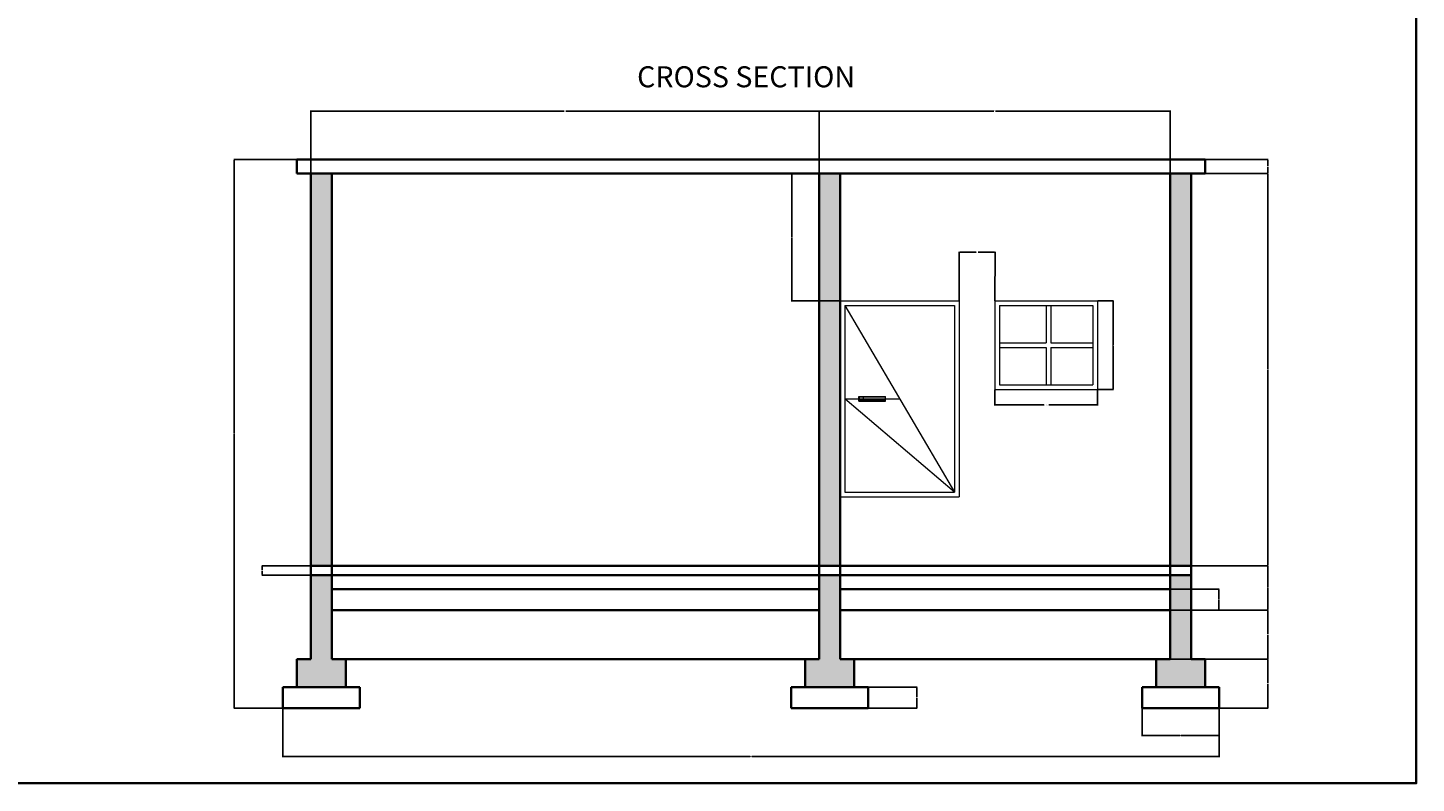
# Model space of a CAD drawing. Units: inches. Extents: x 2473 to 3664, y 1231 to 2079.
# Tile 7 of 8: x 3069 to 3664, y 1231 to 1555. Entities that reach past the tile are written whole.
import ezdxf

# ---------------------------------------------------------------- set-up
doc = ezdxf.new("R2010")
doc.units = ezdxf.units.IN
doc.linetypes.add('ACAD_ISO02W100', pattern=[15, 12, -3])
doc.layers.get('Defpoints').update_dxf_attribs({"linetype": 'ACAD_ISO02W100'})
for name, color, linetype, lineweight in [('A-ANNO-DIMS', 2, 'Continuous', 18), ('A-ANNO-TEXT', 4, 'Continuous', 25), ('A-ANNO-TTLB', 7, 'Continuous', 35), ('A-DOOR', 4, 'Continuous', 18), ('A-GLAZ', 3, 'Continuous', 18), ('A-SECT', 7, 'Continuous', 35), ('A-SECT-PATT', 252, 'Continuous', 13), ('S-FNDN', 7, 'Continuous', 35)]:
    doc.layers.add(name, color=color, linetype=linetype, lineweight=lineweight)
doc.styles.get("Standard").update_dxf_attribs({"font": 'arial.ttf'})
doc.dimstyles.get("Standard").update_dxf_attribs({"dimtxt": 0.18, "dimasz": 0.18, "dimexe": 0.18, "dimexo": 0.0625, "dimgap": 0.09, "dimtad": 0, "dimtih": 1, "dimtoh": 1, "dimdec": 4, "dimzin": 0, "dimdsep": 46, "dimtxsty": 'Standard', "dimcen": 0.09, "dimadec": 0, "dimazin": 0, "dimtfac": 1, "dimtdec": 4, "dimtofl": 0, "dimtmove": 0, "dimatfit": 3, "dimfxl": 1, "dimtolj": 1, "dimtzin": 0, "dimarcsym": 0})

# ---------------------------------------------------------------- blocks, each defined once
blk = doc.blocks.new('DOOR-LEAF-ELEV-47X80')
for p, q in [((0, 80), (47, 80)), ((0, 80), (0, 0)), ((0, 80), (47, 0)), ((47, 80), (47, 0)), ((0, 40), (23.5, 40)), ((47, 0), (0, 40)), ((6.03, 41), (17.47, 41)), ((6.03, 39), (6.03, 41)), ((6.03, 41), (6.33, 40.7)), ((6.03, 39), (6.33, 39.3)), ((6.03, 39), (17.47, 39)), ((17.17, 40.7), (6.33, 40.7)), ((6.33, 39.3), (6.33, 40.7)), ((17.17, 39.3), (6.33, 39.3)), ((8.03, 39.3), (8.03, 40.7)), ((17.47, 41), (17.17, 40.7)), ((17.47, 39), (17.17, 39.3)), ((17.47, 39), (17.47, 41)), ((0, 0), (47, 0))]:
    blk.add_line(p, q)
blk = doc.blocks.new('GLAZ-FOUR-LIGHT-ELEV')
for p, q in [((0, 38), (0, 0)), ((0, 38), (0.02, 38)), ((0.02, 38.03), (44.02, 38.03)), ((2, 36), (2, 2)), ((2, 36), (42.02, 36)), ((22, 36), (22, 20)), ((24, 36), (24, 20)), ((42.02, 36), (42.02, 2)), ((44.02, 38.03), (44.02, 0)), ((2, 20), (22, 20)), ((2, 18), (22, 18)), ((22, 18), (22, 2)), ((24, 20), (42.02, 20)), ((24, 18), (24, 2)), ((24, 18), (42.02, 18)), ((2, 2), (42.02, 2)), ((0, 0), (44.02, 0))]:
    blk.add_line(p, q)
blk = doc.blocks.new('*D31')
at = {"layer": 'A-ANNO-DIMS', "color": 0, "lineweight": -2, "transparency": 16777216}
for p, q in [((3483.19, 1399.9), (3483.19, 1393.18)), ((3527.21, 1399.9), (3527.21, 1393.18)), ((3483.37, 1393.36), (3504.08, 1393.36)), ((3527.03, 1393.36), (3506.32, 1393.36))]:
    blk.add_line(p, q, dxfattribs=at)
at = {"layer": 'A-ANNO-DIMS', "color": 0, "transparency": 16777216}
for points in [[(3483.37, 1393.39), (3483.37, 1393.33), (3483.19, 1393.36)], [(3527.03, 1393.39), (3527.03, 1393.33), (3527.21, 1393.36)]]:
    blk.add_solid(points, dxfattribs=at)
at = {"layer": 'Defpoints', "color": 0, "transparency": 16777216}
for p in [(3483.19, 1399.97), (3527.21, 1399.97), (3527.21, 1393.36)]:
    blk.add_point(p, dxfattribs=at)
at = {"layer": 'A-ANNO-DIMS', "color": 0, "transparency": 16777216, "insert": (3505.2, 1393.36), "char_height": 0.18, "attachment_point": 5}
blk.add_mtext('\\A1;WINDOW 44 TYP.', dxfattribs=at)
blk = doc.blocks.new('*D32')
at = {"layer": 'A-ANNO-DIMS', "color": 0, "lineweight": -2, "transparency": 16777216}
for p, q in [((3527.27, 1438), (3533.99, 1438)), ((3533.81, 1437.82), (3533.81, 1419.17)), ((3533.81, 1400.15), (3533.81, 1418.8)), ((3527.27, 1399.97), (3533.99, 1399.97))]:
    blk.add_line(p, q, dxfattribs=at)
at = {"layer": 'A-ANNO-DIMS', "color": 0, "transparency": 16777216}
for points in [[(3533.78, 1437.82), (3533.84, 1437.82), (3533.81, 1438)], [(3533.78, 1400.15), (3533.84, 1400.15), (3533.81, 1399.97)]]:
    blk.add_solid(points, dxfattribs=at)
at = {"layer": 'Defpoints', "color": 0, "transparency": 16777216}
for p in [(3527.21, 1438), (3533.81, 1438), (3527.21, 1399.97)]:
    blk.add_point(p, dxfattribs=at)
at = {"layer": 'A-ANNO-DIMS', "color": 0, "transparency": 16777216, "insert": (3533.81, 1418.98), "char_height": 0.18, "attachment_point": 5}
blk.add_mtext('\\A1;38 TYP.', dxfattribs=at)
blk = doc.blocks.new('*D90')
at = {"layer": 'A-ANNO-DIMS', "color": 0, "lineweight": -2, "transparency": 16777216}
for p, q in [((3177.86, 1263.42), (3177.86, 1242.5)), ((3579.35, 1263.42), (3579.35, 1242.5)), ((3178.04, 1242.68), (3378.21, 1242.68)), ((3579.17, 1242.68), (3379, 1242.68))]:
    blk.add_line(p, q, dxfattribs=at)
at = {"layer": 'A-ANNO-DIMS', "color": 0, "transparency": 16777216}
for points in [[(3178.04, 1242.71), (3178.04, 1242.65), (3177.86, 1242.68)], [(3579.17, 1242.71), (3579.17, 1242.65), (3579.35, 1242.68)]]:
    blk.add_solid(points, dxfattribs=at)
at = {"layer": 'Defpoints', "color": 0, "transparency": 16777216}
for p in [(3177.86, 1263.48), (3579.35, 1263.48), (3579.35, 1242.68)]:
    blk.add_point(p, dxfattribs=at)
at = {"layer": 'A-ANNO-DIMS', "color": 0, "transparency": 16777216, "insert": (3378.6, 1242.68), "char_height": 0.18, "attachment_point": 5}
blk.add_mtext('\\A1;401.5', dxfattribs=at)
blk = doc.blocks.new('*D91')
at = {"layer": 'A-ANNO-DIMS', "color": 0, "lineweight": -2, "transparency": 16777216}
for p, q in [((3183.79, 1498.48), (3156.88, 1498.48)), ((3157.06, 1498.3), (3157.06, 1381.16)), ((3157.06, 1263.66), (3157.06, 1380.8)), ((3177.79, 1263.48), (3156.88, 1263.48))]:
    blk.add_line(p, q, dxfattribs=at)
at = {"layer": 'A-ANNO-DIMS', "color": 0, "transparency": 16777216}
for points in [[(3157.03, 1498.3), (3157.09, 1498.3), (3157.06, 1498.48)], [(3157.03, 1263.66), (3157.09, 1263.66), (3157.06, 1263.48)]]:
    blk.add_solid(points, dxfattribs=at)
at = {"layer": 'Defpoints', "color": 0, "transparency": 16777216}
for p in [(3157.06, 1498.48), (3183.86, 1498.48), (3177.86, 1263.48)]:
    blk.add_point(p, dxfattribs=at)
at = {"layer": 'A-ANNO-DIMS', "color": 0, "transparency": 16777216, "insert": (3157.06, 1380.98), "char_height": 0.18, "attachment_point": 5}
blk.add_mtext('\\A1;235', dxfattribs=at)
blk = doc.blocks.new('*D92')
at = {"layer": 'A-ANNO-DIMS', "color": 0, "lineweight": -2, "transparency": 16777216}
for p, q in [((3546.35, 1272.42), (3546.35, 1251.5)), ((3579.35, 1272.42), (3579.35, 1251.5)), ((3546.53, 1251.68), (3562.64, 1251.68)), ((3579.17, 1251.68), (3563.07, 1251.68))]:
    blk.add_line(p, q, dxfattribs=at)
at = {"layer": 'A-ANNO-DIMS', "color": 0, "transparency": 16777216}
for points in [[(3546.53, 1251.71), (3546.53, 1251.65), (3546.35, 1251.68)], [(3579.17, 1251.71), (3579.17, 1251.65), (3579.35, 1251.68)]]:
    blk.add_solid(points, dxfattribs=at)
at = {"layer": 'Defpoints', "color": 0, "transparency": 16777216}
for p in [(3546.35, 1272.48), (3579.35, 1272.48), (3546.35, 1251.68)]:
    blk.add_point(p, dxfattribs=at)
at = {"layer": 'A-ANNO-DIMS', "color": 0, "transparency": 16777216, "insert": (3562.85, 1251.68), "char_height": 0.18, "attachment_point": 5}
blk.add_mtext('\\A1;33', dxfattribs=at)
blk = doc.blocks.new('*D93')
at = {"layer": 'A-ANNO-DIMS', "color": 0, "lineweight": -2, "transparency": 16777216}
for p, q in [((3189.86, 1492.54), (3189.86, 1519.46)), ((3190.04, 1519.28), (3298.56, 1519.28)), ((3407.68, 1519.28), (3299.15, 1519.28)), ((3407.86, 1492.54), (3407.86, 1519.46))]:
    blk.add_line(p, q, dxfattribs=at)
at = {"layer": 'A-ANNO-DIMS', "color": 0, "transparency": 16777216}
for points in [[(3190.04, 1519.31), (3190.04, 1519.25), (3189.86, 1519.28)], [(3407.68, 1519.31), (3407.68, 1519.25), (3407.86, 1519.28)]]:
    blk.add_solid(points, dxfattribs=at)
at = {"layer": 'Defpoints', "color": 0, "transparency": 16777216}
for p in [(3407.86, 1519.28), (3189.86, 1492.48), (3407.86, 1492.48)]:
    blk.add_point(p, dxfattribs=at)
at = {"layer": 'A-ANNO-DIMS', "color": 0, "transparency": 16777216, "insert": (3298.86, 1519.28), "char_height": 0.18, "attachment_point": 5}
blk.add_mtext('\\A1;218', dxfattribs=at)
blk = doc.blocks.new('*D94')
at = {"layer": 'A-ANNO-DIMS', "color": 0, "lineweight": -2, "transparency": 16777216}
for p, q in [((3407.86, 1492.54), (3407.86, 1519.46)), ((3408.04, 1519.28), (3482.72, 1519.28)), ((3558.17, 1519.28), (3483.49, 1519.28)), ((3558.35, 1492.54), (3558.35, 1519.46))]:
    blk.add_line(p, q, dxfattribs=at)
at = {"layer": 'A-ANNO-DIMS', "color": 0, "transparency": 16777216}
for points in [[(3408.04, 1519.31), (3408.04, 1519.25), (3407.86, 1519.28)], [(3558.17, 1519.31), (3558.17, 1519.25), (3558.35, 1519.28)]]:
    blk.add_solid(points, dxfattribs=at)
at = {"layer": 'Defpoints', "color": 0, "transparency": 16777216}
for p in [(3558.35, 1519.28), (3407.86, 1492.48), (3558.35, 1492.48)]:
    blk.add_point(p, dxfattribs=at)
at = {"layer": 'A-ANNO-DIMS', "color": 0, "transparency": 16777216, "insert": (3483.1, 1519.28), "char_height": 0.18, "attachment_point": 5}
blk.add_mtext('\\A1;150.5', dxfattribs=at)
blk = doc.blocks.new('*D95')
at = {"layer": 'A-ANNO-DIMS', "color": 0, "lineweight": -2, "transparency": 16777216}
for p, q in [((3567.42, 1492.48), (3600.33, 1492.48)), ((3600.15, 1492.3), (3600.15, 1408.66)), ((3600.15, 1324.66), (3600.15, 1408.3)), ((3567.42, 1324.48), (3600.33, 1324.48))]:
    blk.add_line(p, q, dxfattribs=at)
at = {"layer": 'A-ANNO-DIMS', "color": 0, "transparency": 16777216}
for points in [[(3600.12, 1492.3), (3600.18, 1492.3), (3600.15, 1492.48)], [(3600.12, 1324.66), (3600.18, 1324.66), (3600.15, 1324.48)]]:
    blk.add_solid(points, dxfattribs=at)
at = {"layer": 'Defpoints', "color": 0, "transparency": 16777216}
for p in [(3567.35, 1492.48), (3600.15, 1492.48), (3567.35, 1324.48)]:
    blk.add_point(p, dxfattribs=at)
at = {"layer": 'A-ANNO-DIMS', "color": 0, "transparency": 16777216, "insert": (3600.15, 1408.48), "char_height": 0.18, "attachment_point": 5}
blk.add_mtext('\\A1;168', dxfattribs=at)
blk = doc.blocks.new('*D96')
at = {"layer": 'A-ANNO-DIMS', "color": 0, "lineweight": -2, "transparency": 16777216}
for p, q in [((3573.42, 1498.48), (3600.33, 1498.48)), ((3600.15, 1498.3), (3600.15, 1495.66)), ((3600.15, 1492.66), (3600.15, 1495.3)), ((3573.42, 1492.48), (3600.33, 1492.48))]:
    blk.add_line(p, q, dxfattribs=at)
at = {"layer": 'A-ANNO-DIMS', "color": 0, "transparency": 16777216}
for points in [[(3600.12, 1498.3), (3600.18, 1498.3), (3600.15, 1498.48)], [(3600.12, 1492.66), (3600.18, 1492.66), (3600.15, 1492.48)]]:
    blk.add_solid(points, dxfattribs=at)
at = {"layer": 'Defpoints', "color": 0, "transparency": 16777216}
for p in [(3573.35, 1498.48), (3600.15, 1498.48), (3573.35, 1492.48)]:
    blk.add_point(p, dxfattribs=at)
at = {"layer": 'A-ANNO-DIMS', "color": 0, "transparency": 16777216, "insert": (3600.15, 1495.48), "char_height": 0.18, "attachment_point": 5}
blk.add_mtext('\\A1;6', dxfattribs=at)
blk = doc.blocks.new('*D97')
at = {"layer": 'A-ANNO-DIMS', "color": 0, "lineweight": -2, "transparency": 16777216}
for p, q in [((3573.42, 1284.48), (3600.33, 1284.48)), ((3600.15, 1284.3), (3600.15, 1274.16)), ((3600.15, 1263.66), (3600.15, 1273.8)), ((3579.42, 1263.48), (3600.33, 1263.48))]:
    blk.add_line(p, q, dxfattribs=at)
at = {"layer": 'A-ANNO-DIMS', "color": 0, "transparency": 16777216}
for points in [[(3600.12, 1284.3), (3600.18, 1284.3), (3600.15, 1284.48)], [(3600.12, 1263.66), (3600.18, 1263.66), (3600.15, 1263.48)]]:
    blk.add_solid(points, dxfattribs=at)
at = {"layer": 'Defpoints', "color": 0, "transparency": 16777216}
for p in [(3573.35, 1284.48), (3600.15, 1284.48), (3579.35, 1263.48)]:
    blk.add_point(p, dxfattribs=at)
at = {"layer": 'A-ANNO-DIMS', "color": 0, "transparency": 16777216, "insert": (3600.15, 1273.98), "char_height": 0.18, "attachment_point": 5}
blk.add_mtext('\\A1;21', dxfattribs=at)
blk = doc.blocks.new('*D98')
at = {"layer": 'A-ANNO-DIMS', "color": 0, "lineweight": -2, "transparency": 16777216}
for p, q in [((3428.92, 1272.48), (3449.84, 1272.48)), ((3449.66, 1272.3), (3449.66, 1268.16)), ((3428.92, 1263.48), (3449.84, 1263.48)), ((3449.66, 1263.66), (3449.66, 1267.8))]:
    blk.add_line(p, q, dxfattribs=at)
at = {"layer": 'A-ANNO-DIMS', "color": 0, "transparency": 16777216}
for points in [[(3449.63, 1272.3), (3449.69, 1272.3), (3449.66, 1272.48)], [(3449.63, 1263.66), (3449.69, 1263.66), (3449.66, 1263.48)]]:
    blk.add_solid(points, dxfattribs=at)
at = {"layer": 'Defpoints', "color": 0, "transparency": 16777216}
for p in [(3428.86, 1272.48), (3428.86, 1263.48), (3449.66, 1263.48)]:
    blk.add_point(p, dxfattribs=at)
at = {"layer": 'A-ANNO-DIMS', "color": 0, "transparency": 16777216, "insert": (3449.66, 1267.98), "char_height": 0.18, "attachment_point": 5}
blk.add_mtext('\\A1;9', dxfattribs=at)
blk = doc.blocks.new('*D99')
at = {"layer": 'A-ANNO-DIMS', "color": 0, "lineweight": -2, "transparency": 16777216}
for p, q in [((3416.79, 1492.48), (3395.88, 1492.48)), ((3396.06, 1492.3), (3396.06, 1465.42)), ((3396.06, 1438.18), (3396.06, 1465.06)), ((3416.79, 1438), (3395.88, 1438))]:
    blk.add_line(p, q, dxfattribs=at)
at = {"layer": 'A-ANNO-DIMS', "color": 0, "transparency": 16777216}
for points in [[(3396.03, 1492.3), (3396.09, 1492.3), (3396.06, 1492.48)], [(3396.03, 1438.18), (3396.09, 1438.18), (3396.06, 1438)]]:
    blk.add_solid(points, dxfattribs=at)
at = {"layer": 'Defpoints', "color": 0, "transparency": 16777216}
for p in [(3396.06, 1492.48), (3416.86, 1492.48), (3416.86, 1438)]:
    blk.add_point(p, dxfattribs=at)
at = {"layer": 'A-ANNO-DIMS', "color": 0, "transparency": 16777216, "insert": (3396.06, 1465.24), "char_height": 0.18, "attachment_point": 5}
blk.add_mtext('\\A1;54.48', dxfattribs=at)
blk = doc.blocks.new('*D100')
at = {"layer": 'A-ANNO-DIMS', "color": 0, "lineweight": -2, "transparency": 16777216}
for p, q in [((3467.86, 1438.06), (3467.9, 1458.98)), ((3468.08, 1458.8), (3475.11, 1458.78)), ((3483.05, 1458.77), (3476.02, 1458.78)), ((3483.19, 1438.03), (3483.23, 1458.95))]:
    blk.add_line(p, q, dxfattribs=at)
at = {"layer": 'A-ANNO-DIMS', "color": 0, "transparency": 16777216}
for points in [[(3468.08, 1458.83), (3468.08, 1458.77), (3467.9, 1458.8)], [(3483.05, 1458.8), (3483.05, 1458.74), (3483.23, 1458.77)]]:
    blk.add_solid(points, dxfattribs=at)
at = {"layer": 'Defpoints', "color": 0, "transparency": 16777216}
for p in [(3483.23, 1458.77), (3467.86, 1438), (3483.19, 1437.97)]:
    blk.add_point(p, dxfattribs=at)
at = {"layer": 'A-ANNO-DIMS', "color": 0, "transparency": 16777216, "insert": (3475.57, 1458.78), "char_height": 0.18, "attachment_point": 5}
blk.add_mtext('\\A1;15.333', dxfattribs=at)
blk = doc.blocks.new('*D101')
at = {"layer": 'A-ANNO-DIMS', "color": 0, "lineweight": -2, "transparency": 16777216}
for p, q in [((3558.42, 1305.48), (3600.33, 1305.48)), ((3600.15, 1305.3), (3600.15, 1295.16)), ((3600.15, 1284.66), (3600.15, 1294.8)), ((3552.42, 1284.48), (3600.33, 1284.48))]:
    blk.add_line(p, q, dxfattribs=at)
at = {"layer": 'A-ANNO-DIMS', "color": 0, "transparency": 16777216}
for points in [[(3600.12, 1305.3), (3600.18, 1305.3), (3600.15, 1305.48)], [(3600.12, 1284.66), (3600.18, 1284.66), (3600.15, 1284.48)]]:
    blk.add_solid(points, dxfattribs=at)
at = {"layer": 'Defpoints', "color": 0, "transparency": 16777216}
for p in [(3558.35, 1305.48), (3600.15, 1305.48), (3552.35, 1284.48)]:
    blk.add_point(p, dxfattribs=at)
at = {"layer": 'A-ANNO-DIMS', "color": 0, "transparency": 16777216, "insert": (3600.15, 1294.98), "char_height": 0.18, "attachment_point": 5}
blk.add_mtext('\\A1;21', dxfattribs=at)
blk = doc.blocks.new('*D102')
at = {"layer": 'A-ANNO-DIMS', "color": 0, "lineweight": -2, "transparency": 16777216}
for p, q in [((3567.42, 1324.48), (3600.33, 1324.48)), ((3600.15, 1324.3), (3600.15, 1315.16)), ((3600.15, 1305.66), (3600.15, 1314.8)), ((3558.42, 1305.48), (3600.33, 1305.48))]:
    blk.add_line(p, q, dxfattribs=at)
at = {"layer": 'A-ANNO-DIMS', "color": 0, "transparency": 16777216}
for points in [[(3600.12, 1324.3), (3600.18, 1324.3), (3600.15, 1324.48)], [(3600.12, 1305.66), (3600.18, 1305.66), (3600.15, 1305.48)]]:
    blk.add_solid(points, dxfattribs=at)
at = {"layer": 'Defpoints', "color": 0, "transparency": 16777216}
for p in [(3567.35, 1324.48), (3600.15, 1324.48), (3558.35, 1305.48)]:
    blk.add_point(p, dxfattribs=at)
at = {"layer": 'A-ANNO-DIMS', "color": 0, "transparency": 16777216, "insert": (3600.15, 1314.98), "char_height": 0.18, "attachment_point": 5}
blk.add_mtext('\\A1;19', dxfattribs=at)
blk = doc.blocks.new('*D103')
at = {"layer": 'A-ANNO-DIMS', "color": 0, "lineweight": -2, "transparency": 16777216}
for p, q in [((3558.42, 1314.48), (3579.33, 1314.48)), ((3579.15, 1314.3), (3579.15, 1310.16)), ((3579.15, 1305.66), (3579.15, 1309.8)), ((3558.42, 1305.48), (3579.33, 1305.48))]:
    blk.add_line(p, q, dxfattribs=at)
at = {"layer": 'A-ANNO-DIMS', "color": 0, "transparency": 16777216}
for points in [[(3579.12, 1314.3), (3579.18, 1314.3), (3579.15, 1314.48)], [(3579.12, 1305.66), (3579.18, 1305.66), (3579.15, 1305.48)]]:
    blk.add_solid(points, dxfattribs=at)
at = {"layer": 'Defpoints', "color": 0, "transparency": 16777216}
for p in [(3558.35, 1314.48), (3558.35, 1305.48), (3579.15, 1305.48)]:
    blk.add_point(p, dxfattribs=at)
at = {"layer": 'A-ANNO-DIMS', "color": 0, "transparency": 16777216, "insert": (3579.15, 1309.98), "char_height": 0.18, "attachment_point": 5}
blk.add_mtext('\\A1;9', dxfattribs=at)
blk = doc.blocks.new('*D104')
at = {"layer": 'A-ANNO-DIMS', "color": 0, "lineweight": -2, "transparency": 16777216}
for p, q in [((3189.792531, 1324.479738), (3168.875031, 1324.479738)), ((3169.055031, 1324.299738), (3169.055031, 1322.659738)), ((3169.055031, 1320.659738), (3169.055031, 1322.299738)), ((3189.792531, 1320.479738), (3168.875031, 1320.479738))]:
    blk.add_line(p, q, dxfattribs=at)
at = {"layer": 'A-ANNO-DIMS', "color": 0, "transparency": 16777216}
for points in [[(3169.025031, 1324.299738), (3169.085031, 1324.299738), (3169.055031, 1324.479738)], [(3169.025031, 1320.659738), (3169.085031, 1320.659738), (3169.055031, 1320.479738)]]:
    blk.add_solid(points, dxfattribs=at)
at = {"layer": 'Defpoints', "color": 0, "transparency": 16777216}
for p in [(3169.055031, 1324.479738), (3189.855031, 1324.479738), (3189.855031, 1320.479738)]:
    blk.add_point(p, dxfattribs=at)
at = {"layer": 'A-ANNO-DIMS', "color": 0, "transparency": 16777216, "insert": (3169.055031, 1322.479738), "char_height": 0.18, "attachment_point": 5}
blk.add_mtext('\\A1;4', dxfattribs=at)

msp = doc.modelspace()

# ---------------------------------------------------------------- hatches: boundary and pattern name
at = {"layer": 'A-SECT-PATT'}
h = msp.add_hatch(dxfattribs=at)
h.set_pattern_fill('AR-RROOF', color=256)
h.set_pattern_definition([(0, (572.195, 296.425), (55.88, 25.4), [381, -50.8, 127, -25.4]), (0, (605.977, 309.125), (-25.4, 33.782), [76.2, -8.382, 152.4, -19.05]), (0, (584.895, 318.015), (132.08, 17.018), [203.2, -35.56, 101.6, -25.4])])
h.paths.add_polyline_path([(3183.855, 1498.4797), (3183.855, 1492.4797), (3189.855, 1492.4797), (3573.354, 1492.4797), (3573.354, 1498.4797)])
h = msp.add_hatch(dxfattribs=at)
h.set_pattern_fill('ANSI36', color=256)
h.set_pattern_definition([(45, (572.1946, 296.4252), (1.683798, 6.173926), [7.9375, -1.5875, 0, -1.5875])])
h.paths.add_polyline_path([(3198.855, 1492.4797), (3189.855, 1492.4797), (3189.855, 1324.4797), (3198.855, 1324.4797)])
h.paths.add_polyline_path([(3407.855, 1324.4797), (3416.855, 1324.4797), (3416.855, 1492.4797), (3407.855, 1492.4797)])
h.paths.add_polyline_path([(3558.354, 1324.4797), (3567.354, 1324.4797), (3567.354, 1492.4797), (3558.354, 1492.4797)])
h.paths.add_polyline_path([(3198.855, 1320.4797), (3189.855, 1320.4797), (3189.855, 1284.4797), (3183.855, 1284.4797), (3183.855, 1272.4797), (3204.855, 1272.4797), (3204.855, 1284.4797), (3198.855, 1284.4797)])
h.paths.add_polyline_path([(3407.855, 1284.4797), (3401.855, 1284.4797), (3401.855, 1272.4797), (3422.855, 1272.4797), (3422.855, 1284.4797), (3416.855, 1284.4797), (3416.855, 1320.4797), (3407.855, 1320.4797)])
h.paths.add_polyline_path([(3558.354, 1284.4797), (3552.354, 1284.4797), (3552.354, 1272.4797), (3573.354, 1272.4797), (3573.354, 1284.4797), (3567.354, 1284.4797), (3567.354, 1320.4797), (3558.354, 1320.4797)])

# ---------------------------------------------------------------- linework, layer by layer
at = {"layer": 'A-ANNO-TTLB'}
msp.add_lwpolyline([(2473.2801, 2079.0861), (3663.7983, 2079.0861), (3663.7983, 1231.3065), (2473.2801, 1231.3065)], close=True, dxfattribs=at)
at = {"layer": 'A-DOOR'}
for p, q in [((3416.855, 1437.9995), (3467.855, 1437.9995)), ((3467.855, 1437.9995), (3467.855, 1353.9995)), ((3416.855, 1353.9995), (3467.855, 1353.9995))]:
    msp.add_line(p, q, dxfattribs=at)
at = {"layer": 'A-SECT'}
for p, q in [((3183.855, 1498.4797), (3573.354, 1498.4797)), ((3183.855, 1498.4797), (3183.855, 1492.4797)), ((3573.354, 1498.4797), (3573.354, 1492.4797)), ((3183.855, 1492.4797), (3189.855, 1492.4797)), ((3189.855, 1492.4797), (3189.855, 1284.4797)), ((3189.855, 1492.4797), (3573.354, 1492.4797)), ((3198.855, 1492.4797), (3198.855, 1284.4797)), ((3407.855, 1492.4797), (3407.855, 1284.4797)), ((3416.855, 1492.4797), (3416.855, 1284.4797)), ((3558.354, 1492.4797), (3558.354, 1284.4797)), ((3567.354, 1492.4797), (3567.354, 1284.4797)), ((3189.855, 1324.4797), (3567.354, 1324.4797)), ((3189.855, 1320.4797), (3567.354, 1320.4797)), ((3198.855, 1314.4797), (3407.855, 1314.4797)), ((3416.855, 1314.4797), (3558.354, 1314.4797)), ((3198.855, 1305.4797), (3407.855, 1305.4797)), ((3416.855, 1305.4797), (3558.354, 1305.4797)), ((3198.855, 1284.4797), (3407.855, 1284.4797)), ((3416.855, 1284.4797), (3558.354, 1284.4797))]:
    msp.add_line(p, q, dxfattribs=at)
at = {"layer": 'S-FNDN'}
for p, q in [((3183.855, 1284.4797), (3183.855, 1272.4797)), ((3183.855, 1284.4797), (3189.855, 1284.4797)), ((3204.855, 1284.4797), (3198.855, 1284.4797)), ((3204.855, 1284.4797), (3204.855, 1272.4797)), ((3401.855, 1284.4797), (3401.855, 1272.4797)), ((3401.855, 1284.4797), (3407.855, 1284.4797)), ((3422.855, 1284.4797), (3416.855, 1284.4797)), ((3422.855, 1284.4797), (3422.855, 1272.4797)), ((3552.354, 1284.4797), (3552.354, 1272.4797)), ((3552.354, 1284.4797), (3558.354, 1284.4797)), ((3573.354, 1284.4797), (3567.354, 1284.4797)), ((3573.354, 1284.4797), (3573.354, 1272.4797)), ((3177.855, 1272.4797), (3183.855, 1272.4797)), ((3177.855, 1272.4797), (3177.855, 1263.4797)), ((3183.855, 1272.4797), (3204.855, 1272.4797)), ((3204.855, 1272.4797), (3210.855, 1272.4797)), ((3210.855, 1272.4797), (3210.855, 1263.4797)), ((3395.855, 1272.4797), (3395.855, 1263.4797)), ((3395.855, 1272.4797), (3401.855, 1272.4797)), ((3401.855, 1272.4797), (3422.855, 1272.4797)), ((3422.855, 1272.4797), (3428.855, 1272.4797)), ((3428.855, 1272.4797), (3428.855, 1263.4797)), ((3546.354, 1272.4797), (3546.354, 1263.4797)), ((3546.354, 1272.4797), (3552.354, 1272.4797)), ((3552.354, 1272.4797), (3573.354, 1272.4797)), ((3573.354, 1272.4797), (3579.354, 1272.4797)), ((3579.354, 1272.4797), (3579.354, 1263.4797)), ((3177.855, 1263.4797), (3210.855, 1263.4797)), ((3395.855, 1263.4797), (3428.855, 1263.4797)), ((3546.354, 1263.4797), (3579.354, 1263.4797))]:
    msp.add_line(p, q, dxfattribs=at)

# ---------------------------------------------------------------- block references
at = {"layer": 'A-DOOR'}
msp.add_blockref('DOOR-LEAF-ELEV-47X80', (3418.8546, 1355.9993), dxfattribs=at)
at = {"layer": 'A-GLAZ'}
msp.add_blockref('GLAZ-FOUR-LIGHT-ELEV', (3483.1886, 1399.9673), dxfattribs=at)

# ---------------------------------------------------------------- texts
at = {"layer": 'A-ANNO-TEXT'}
msp.add_text('CROSS SECTION', height=9, dxfattribs=at).set_placement((3329.7718, 1529.453))

# ---------------------------------------------------------------- dimensions: what is measured, and where the dimension line sits
at = {"layer": 'A-ANNO-DIMS'}
for base, p1, p2, override, picture, middle in [((3407.855, 1519.2797), (3189.855, 1492.4797), (3407.855, 1492.4797), {"dimdec": 0, "dimlfac": 1, "dimrnd": 0, "dimzin": 0, "dimdsep": 46, "dimlunit": 2}, '*D93', (3298.855, 1519.2797)), ((3558.354, 1519.2797), (3407.855, 1492.4797), (3558.354, 1492.4797), {"dimdec": 1, "dimlfac": 1, "dimrnd": 0, "dimzin": 0, "dimdsep": 46, "dimlunit": 2}, '*D94', (3483.1045, 1519.2797)), ((3579.354, 1242.6797), (3177.855, 1263.4797), (3579.354, 1263.4797), {"dimdec": 1, "dimlfac": 1, "dimrnd": 0, "dimzin": 0, "dimdsep": 46, "dimlunit": 2}, '*D90', (3378.6045, 1242.6797))]:
    dim = msp.add_linear_dim(base=base, p1=p1, p2=p2, dimstyle='Standard', override=override, dxfattribs=at)
    dim.commit()
    dim.dimension.update_dxf_attribs({"geometry": picture, "text_midpoint": middle})
for base, p1, p2, angle, override, picture, middle in [((3157.055, 1498.4797), (3177.855, 1263.4797), (3183.855, 1498.4797), 90, {"dimdec": 0, "dimlfac": 1, "dimrnd": 0, "dimzin": 0, "dimdsep": 46, "dimlunit": 2}, '*D91', (3157.055, 1380.9797)), ((3600.154, 1498.4797), (3573.354, 1492.4797), (3573.354, 1498.4797), 90, {"dimdec": 0, "dimlfac": 1, "dimrnd": 0, "dimzin": 0, "dimdsep": 46, "dimlunit": 2}, '*D96', (3600.154, 1495.4797)), ((3396.055, 1492.4797), (3416.855, 1437.9995), (3416.855, 1492.4797), 90, {"dimdec": 2, "dimlfac": 1, "dimrnd": 0, "dimzin": 0, "dimdsep": 46, "dimlunit": 2}, '*D99', (3396.055, 1465.2396)), ((3600.154, 1492.4797), (3567.354, 1324.4797), (3567.354, 1492.4797), 90, {"dimdec": 0, "dimlfac": 1, "dimrnd": 0, "dimzin": 0, "dimdsep": 46, "dimlunit": 2}, '*D95', (3600.154, 1408.4797)), ((3483.2322, 1458.7671), (3467.855, 1437.9995), (3483.1883, 1437.9671), 359.8790754, {"dimdec": 3, "dimlfac": 1, "dimrnd": 0, "dimzin": 0, "dimdsep": 46, "dimlunit": 2}, '*D100', (3475.5656, 1458.7832)), ((3169.055, 1324.4797), (3189.855, 1320.4797), (3189.855, 1324.4797), 90, {"dimdec": 0, "dimlfac": 1, "dimrnd": 0, "dimzin": 0, "dimdsep": 46, "dimlunit": 2}, '*D104', (3169.055, 1322.4797)), ((3600.154, 1324.4797), (3558.354, 1305.4797), (3567.354, 1324.4797), 90, {"dimdec": 0, "dimlfac": 1, "dimrnd": 0, "dimzin": 0, "dimdsep": 46, "dimlunit": 2}, '*D102', (3600.154, 1314.9797)), ((3579.154, 1305.4797), (3558.354, 1314.4797), (3558.354, 1305.4797), 270, {"dimdec": 0, "dimlfac": 1, "dimrnd": 0, "dimzin": 0, "dimdsep": 46, "dimlunit": 2}, '*D103', (3579.154, 1309.9797)), ((3600.154, 1305.4797), (3552.354, 1284.4797), (3558.354, 1305.4797), 90, {"dimdec": 0, "dimlfac": 1, "dimrnd": 0, "dimzin": 0, "dimdsep": 46, "dimlunit": 2}, '*D101', (3600.154, 1294.9797)), ((3600.154, 1284.4797), (3579.354, 1263.4797), (3573.354, 1284.4797), 90, {"dimdec": 0, "dimlfac": 1, "dimrnd": 0, "dimzin": 0, "dimdsep": 46, "dimlunit": 2}, '*D97', (3600.154, 1273.9797)), ((3449.655, 1263.4797), (3428.855, 1272.4797), (3428.855, 1263.4797), 270, {"dimdec": 0, "dimlfac": 1, "dimrnd": 0, "dimzin": 0, "dimdsep": 46, "dimlunit": 2}, '*D98', (3449.655, 1267.9797)), ((3546.354, 1251.6797), (3579.354, 1272.4797), (3546.354, 1272.4797), 180, {"dimdec": 0, "dimlfac": 1, "dimrnd": 0, "dimzin": 0, "dimdsep": 46, "dimlunit": 2}, '*D92', (3562.854, 1251.6797))]:
    dim = msp.add_linear_dim(base=base, p1=p1, p2=p2, angle=angle, dimstyle='Standard', override=override, dxfattribs=at)
    dim.commit()
    dim.dimension.update_dxf_attribs({"geometry": picture, "text_midpoint": middle})
dim = msp.add_linear_dim(base=(3533.8107, 1437.9995), p1=(3527.2077, 1399.9671), p2=(3527.2077, 1437.9995), angle=90, text='<> TYP.', dimstyle='Standard', override={"dimdec": 0, "dimlfac": 1, "dimrnd": 0, "dimzin": 0, "dimdsep": 46, "dimlunit": 2}, dxfattribs=at)
dim.commit()
dim.dimension.update_dxf_attribs({"geometry": '*D32', "text_midpoint": (3533.8107, 1418.9833)})
dim = msp.add_linear_dim(base=(3527.2077, 1393.3642), p1=(3483.1883, 1399.9671), p2=(3527.2077, 1399.9671), text='WINDOW <> TYP.', dimstyle='Standard', override={"dimdec": 0, "dimlfac": 1, "dimrnd": 0, "dimzin": 0, "dimdsep": 46, "dimlunit": 2}, dxfattribs=at)
dim.commit()
dim.dimension.update_dxf_attribs({"geometry": '*D31', "text_midpoint": (3505.198, 1393.3642)})

doc.saveas('drawing.dxf')
